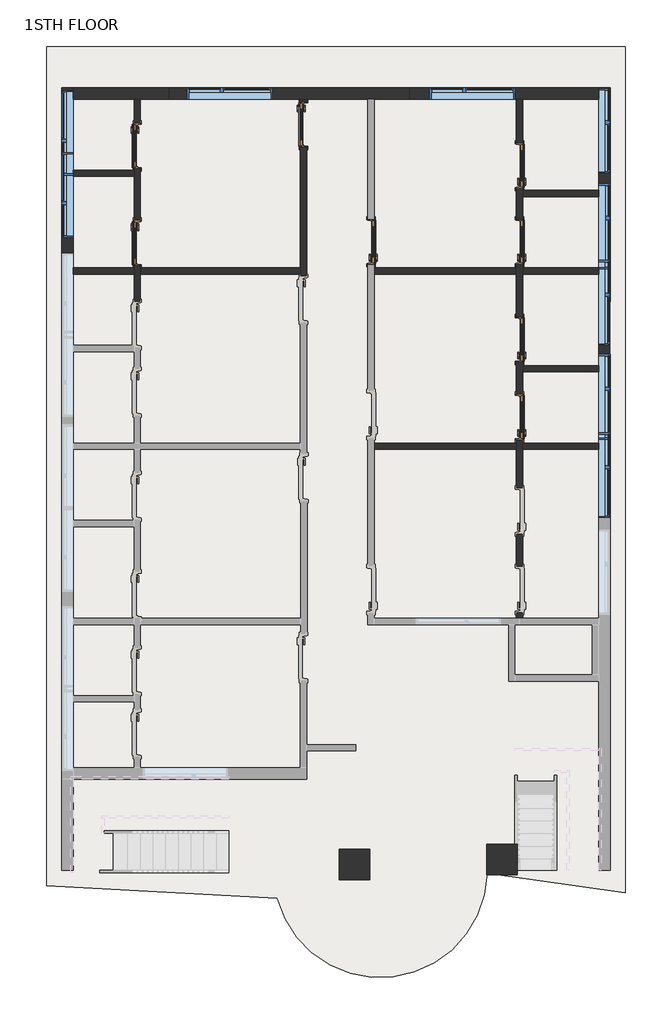
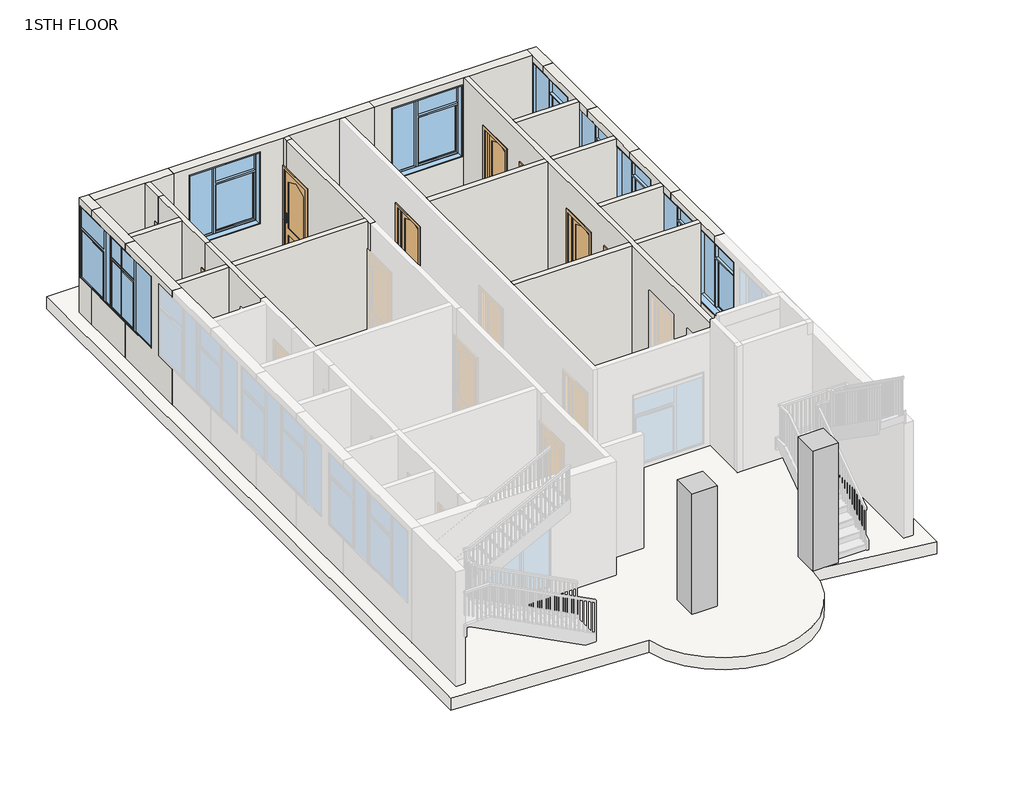
# One storey, part 2 of 4: 26 walls, 9 windows, 8 doors, 2 columns, 1 slab.
"""IFC4 building model written with IfcOpenShell, lengths in millimetres."""

from ifc_helpers import new_model, si_unit, point, frame, frame_2d, origin, place, context, project, spatial, polyline, circle_curve, trimmed, segment, composite_curve, outline, extrude, faceted_brep, transform, mapped, element, save
from components import column_8afb6978, door_346b4a94, m_window_casement_double_sidelight_1702_x_1829mm_c8b42c7f

model = new_model("IFC4")

# Units and contexts
model_context = context("Model", 3, world=origin())
ifc_project = project(units=[si_unit("LENGTHUNIT", "METRE", prefix="MILLI")], contexts=[model_context])

# Site, building, storey
site = spatial("IfcSite", under=ifc_project)
building = spatial("IfcBuilding", under=site)
storey = spatial("IfcBuildingStorey", under=building, Name="1STH FLOOR", Elevation=3200.4)

# Columns
placement = place(None, origin())
element("IfcColumn", 1, ObjectType="Rectangular Column : 24\" x 24\"", at=placement, inside=storey, context=model_context, shape_type="SweptSolid", body=[
    extrude(outline(polyline([(2657.4891134, -7132.8082131), (2657.4891134, -7742.4082131), (2047.8891134, -7742.4082131), (2047.8891134, -7132.8082131), (2657.4891134, -7132.8082131)])), frame((0.0, 0.0, 3200.4), z_axis=(0.0, 0.0, 1.0), x_axis=(1.0, 0.0, 0.0)), (0.0, 0.0, 1.0), 3048.0),
])
column_shape = column_8afb6978(model_context)
element("IfcColumn", 2, ObjectType="Rectangular Column : 24\" x 24\"", at=placement, inside=storey, context=model_context, shape_type="MappedRepresentation", body=[
    mapped(column_shape, transform((-606.4108866, -7539.2082131, 0.0), x_axis=(1.0, 0.0, 0.0), y_axis=(0.0, 1.0, 0.0), z_axis=(0.0, 0.0, 1.0))),
])

# Doors
door_shape = door_346b4a94(model_context)
element("IfcDoor", 3, ObjectType="2'10\"X7'", at=placement, inside=storey, context=model_context, shape_type="MappedRepresentation", body=[
    mapped(door_shape, transform((2698.7641134, 6449.4399728, 3200.4), x_axis=(0.0, -1.0, 0.0), y_axis=(1.0, 0.0, 0.0), z_axis=(0.0, 0.0, 1.0))),
])
element("IfcDoor", 4, ObjectType="2'10\"X7'", at=placement, inside=storey, context=model_context, shape_type="MappedRepresentation", body=[
    mapped(door_shape, transform((2698.7641134, 4925.4399728, 3200.4), x_axis=(0.0, -1.0, 0.0), y_axis=(1.0, 0.0, 0.0), z_axis=(0.0, 0.0, 1.0))),
])
element("IfcDoor", 5, ObjectType="2'10\"X7'", at=placement, inside=storey, context=model_context, shape_type="MappedRepresentation", body=[
    mapped(door_shape, transform((2698.7641134, 2969.6399728, 3200.4), x_axis=(0.0, -1.0, 0.0), y_axis=(1.0, 0.0, 0.0), z_axis=(0.0, 0.0, 1.0))),
])
element("IfcDoor", 6, ObjectType="2'10\"X7'", at=placement, inside=storey, context=model_context, shape_type="MappedRepresentation", body=[
    mapped(door_shape, transform((2698.7641134, 1420.2399728, 3200.4), x_axis=(0.0, -1.0, 0.0), y_axis=(1.0, 0.0, 0.0), z_axis=(0.0, 0.0, 1.0))),
])
element("IfcDoor", 7, ObjectType="2'10\"X7'", at=placement, inside=storey, context=model_context, shape_type="MappedRepresentation", body=[
    mapped(door_shape, transform((-273.0358866, 4925.4399728, 3200.4), x_axis=(0.0, -1.0, 0.0), y_axis=(1.0, 0.0, 0.0), z_axis=(0.0, 0.0, 1.0))),
])
element("IfcDoor", 8, ObjectType="2'10\"X7'", at=placement, inside=storey, context=model_context, shape_type="MappedRepresentation", body=[
    mapped(door_shape, transform((-4952.9858866, 4900.320652, 3200.4), x_axis=(0.0, 1.0, 0.0), y_axis=(-1.0, 0.0, 0.0), z_axis=(0.0, 0.0, 1.0))),
])
element("IfcDoor", 9, ObjectType="2'10\"X7'", at=placement, inside=storey, context=model_context, shape_type="MappedRepresentation", body=[
    mapped(door_shape, transform((-4952.9858866, 6843.9929737, 3200.4), x_axis=(0.0, 1.0, 0.0), y_axis=(-1.0, 0.0, 0.0), z_axis=(0.0, 0.0, 1.0))),
])
element("IfcDoor", 10, ObjectType="2'10\"X7'", at=placement, inside=storey, context=model_context, shape_type="MappedRepresentation", body=[
    mapped(door_shape, transform((-1625.5858866, 7274.3310623, 3200.4), x_axis=(0.0, 1.0, 0.0), y_axis=(-1.0, 0.0, 0.0), z_axis=(0.0, 0.0, 1.0))),
])

# Slab
element("IfcSlab", 11, ObjectType="Generic - 12\"", at=placement, inside=storey, context=model_context, shape_type="SweptSolid", body=[
    extrude(outline(composite_curve([segment(polyline([(4815.1311655, 8833.6177996), (4815.1311655, -8095.4822004), (2048.5236178, -7706.6608663)]), True, "CONTINUOUS"), segment(trimmed(circle_curve(frame_2d((-85.9459984, -7660.7851902)), 2134.962557), [point((2048.5236178, -7706.6608663))], [point((-2148.0488767, -8213.7741944))], False, "CARTESIAN"), True, "CONTINUOUS"), segment(polyline([(-2148.0488767, -8213.7741944), (-6765.9108866, -7964.6582131), (-6765.9108866, 8833.6177996), (4815.1311655, 8833.6177996)]), True, "CONTINUOUS")], self_intersect=False)), frame((0.0, 0.0, 2895.6), z_axis=(0.0, 0.0, 1.0), x_axis=(1.0, 0.0, 0.0)), (0.0, 0.0, 1.0), 304.8),
])

# Walls
element("IfcWall", 12, ObjectType="Generic - 4.5\"", at=placement, inside=storey, context=model_context, shape_type="SweptSolid", body=[
    extrude(outline(polyline([(7782.9399728, 6096.0), (7782.9399728, 3200.4), (7300.7929737, 3200.4), (7300.7929737, 5359.0), (7224.9929737, 5359.0), (7224.9929737, 6096.0), (7782.9399728, 6096.0)])), frame((-5013.3108866, 0.0, 0.0), z_axis=(1.0, 0.0, 0.0), x_axis=(0.0, 1.0, 0.0)), (0.0, 0.0, 1.0), 127.0),
])
element("IfcWall", 13, ObjectType="Generic - 4.5\"", at=placement, inside=storey, context=model_context, shape_type="Brep", body=[
    faceted_brep([(-5013.3108866, 5281.320652, 5359.0), (-5013.3108866, 5281.320652, 6096.0), (-5013.3108866, 6233.5399728, 6096.0), (-5013.3108866, 6360.5399728, 6096.0), (-5013.3108866, 7224.9929737, 6096.0), (-5013.3108866, 7224.9929737, 5359.0), (-5013.3108866, 6387.1929737, 5359.0), (-5013.3108866, 6387.1929737, 3200.4), (-5013.3108866, 6360.5399728, 3200.4), (-5013.3108866, 6233.5399728, 3200.4), (-5013.3108866, 5357.120652, 3200.4), (-5013.3108866, 5357.120652, 5359.0), (-4886.3108866, 5281.320652, 6096.0), (-4886.3108866, 5281.320652, 5359.0), (-4886.3108866, 5357.120652, 5359.0), (-4886.3108866, 5357.120652, 3200.4), (-4886.3108866, 6387.1929737, 3200.4), (-4886.3108866, 6387.1929737, 5359.0), (-4886.3108866, 7224.9929737, 5359.0), (-4886.3108866, 7224.9929737, 6096.0)], [[[0, 1, 2, 3, 4, 5, 6, 7, 8, 9, 10, 11]], [[12, 13, 14, 15, 16, 17, 18, 19]], [[15, 10, 9, 8, 7, 16]], [[1, 0, 13, 12]], [[4, 19, 18, 5]], [[14, 11, 10, 15]], [[11, 14, 13, 0]], [[17, 6, 5, 18]], [[6, 17, 16, 7]], [[4, 3, 2, 1, 12, 19]]]),
])
element("IfcWall", 14, ObjectType="Generic - 4.5\"", at=placement, inside=storey, context=model_context, shape_type="SweptSolid", body=[
    extrude(outline(polyline([(-5013.3108866, 6233.5399728), (-6232.5508078, 6233.5399728), (-6232.5508078, 6360.5399728), (-5013.3108866, 6360.5399728), (-5013.3108866, 6233.5399728)])), frame((0.0, 0.0, 3200.4), z_axis=(0.0, 0.0, 1.0), x_axis=(1.0, 0.0, 0.0)), (0.0, 0.0, 1.0), 2895.6),
])
element("IfcWall", 15, ObjectType="Generic - 4.5\"", at=placement, inside=storey, context=model_context, shape_type="SweptSolid", body=[
    extrude(outline(polyline([(-5013.3108866, 4277.7399728), (-6232.5508078, 4277.7399728), (-6232.5508078, 4404.7399728), (-5013.3108866, 4404.7399728), (-5013.3108866, 4277.7399728)])), frame((0.0, 0.0, 3200.4), z_axis=(0.0, 0.0, 1.0), x_axis=(1.0, 0.0, 0.0)), (0.0, 0.0, 1.0), 2895.6),
])
element("IfcWall", 16, ObjectType="Generic - 4.5\"", at=placement, inside=storey, context=model_context, shape_type="Brep", body=[
    faceted_brep([(-5013.3108866, 2968.8174518, 5359.0), (-5013.3108866, 2968.8174518, 6096.0), (-5013.3108866, 4277.7399728, 6096.0), (-5013.3108866, 4404.7399728, 6096.0), (-5013.3108866, 5281.320652, 6096.0), (-5013.3108866, 5281.320652, 5359.0), (-5013.3108866, 4443.520652, 5359.0), (-5013.3108866, 4443.520652, 3200.4), (-5013.3108866, 4404.7399728, 3200.4), (-5013.3108866, 4277.7399728, 3200.4), (-5013.3108866, 3730.4174518, 3200.4), (-5013.3108866, 3730.4174518, 5359.0), (-4886.3108866, 2968.8174518, 6096.0), (-4886.3108866, 2968.8174518, 5359.0), (-4886.3108866, 3730.4174518, 5359.0), (-4886.3108866, 3730.4174518, 3200.4), (-4886.3108866, 4277.7399728, 3200.4), (-4886.3108866, 4404.7399728, 3200.4), (-4886.3108866, 4443.520652, 3200.4), (-4886.3108866, 4443.520652, 5359.0), (-4886.3108866, 5281.320652, 5359.0), (-4886.3108866, 5281.320652, 6096.0), (-4886.3108866, 4404.7399728, 6096.0), (-4886.3108866, 4277.7399728, 6096.0)], [[[0, 1, 2, 3, 4, 5, 6, 7, 8, 9, 10, 11]], [[12, 13, 14, 15, 16, 17, 18, 19, 20, 21, 22, 23]], [[15, 10, 9, 8, 7, 18, 17, 16]], [[1, 0, 13, 12]], [[4, 21, 20, 5]], [[14, 11, 10, 15]], [[11, 14, 13, 0]], [[19, 6, 5, 20]], [[6, 19, 18, 7]], [[4, 3, 2, 1, 12, 23, 22, 21]]]),
])
element("IfcWall", 17, ObjectType="Generic - 4.5\"", at=placement, inside=storey, context=model_context, shape_type="SweptSolid", body=[
    extrude(outline(polyline([(-1685.9108866, 4277.7399728), (-4886.3108866, 4277.7399728), (-4886.3108866, 4404.7399728), (-1685.9108866, 4404.7399728), (-1685.9108866, 4277.7399728)])), frame((0.0, 0.0, 3200.4), z_axis=(0.0, 0.0, 1.0), x_axis=(1.0, 0.0, 0.0)), (0.0, 0.0, 1.0), 2895.6),
])
element("IfcWall", 18, ObjectType="Generic - 4.5\"", at=placement, inside=storey, context=model_context, shape_type="SweptSolid", body=[
    extrude(outline(polyline([(7782.9399728, 6096.0), (7782.9399728, 3200.4), (7731.1310623, 3200.4), (7731.1310623, 5359.0), (7655.3310623, 5359.0), (7655.3310623, 6096.0), (7782.9399728, 6096.0)])), frame((-1685.9108866, 0.0, 0.0), z_axis=(1.0, 0.0, 0.0), x_axis=(0.0, 1.0, 0.0)), (0.0, 0.0, 1.0), 127.0),
])
element("IfcWall", 19, ObjectType="Generic - 4.5\"", at=placement, inside=storey, context=model_context, shape_type="Brep", body=[
    faceted_brep([(-1685.9108866, 4182.2008884, 5359.0), (-1685.9108866, 4182.2008884, 6096.0), (-1685.9108866, 4277.7399728, 6096.0), (-1685.9108866, 4404.7399728, 6096.0), (-1685.9108866, 7655.3310623, 6096.0), (-1685.9108866, 7655.3310623, 5359.0), (-1685.9108866, 6817.5310623, 5359.0), (-1685.9108866, 6817.5310623, 3200.4), (-1685.9108866, 4404.7399728, 3200.4), (-1685.9108866, 4277.7399728, 3200.4), (-1685.9108866, 4232.6008884, 3200.4), (-1685.9108866, 4232.6008884, 5359.0), (-1558.9108866, 4182.2008884, 6096.0), (-1558.9108866, 4182.2008884, 5359.0), (-1558.9108866, 4232.6008884, 5359.0), (-1558.9108866, 4232.6008884, 3200.4), (-1558.9108866, 6817.5310623, 3200.4), (-1558.9108866, 6817.5310623, 5359.0), (-1558.9108866, 7655.3310623, 5359.0), (-1558.9108866, 7655.3310623, 6096.0), (-1685.4871817, 4182.2008884, 5359.0), (-1685.4871817, 4182.2008884, 6096.0)], [[[0, 1, 2, 3, 4, 5, 6, 7, 8, 9, 10, 11]], [[12, 13, 14, 15, 16, 17, 18, 19]], [[15, 10, 9, 8, 7, 16]], [[1, 0, 20, 13, 12, 21]], [[4, 19, 18, 5]], [[14, 11, 10, 15]], [[11, 14, 13, 20, 0]], [[17, 6, 5, 18]], [[6, 17, 16, 7]], [[4, 3, 2, 1, 21, 12, 19]]]),
])
element("IfcWall", 20, ObjectType="Generic - 4.5\"", at=placement, inside=storey, context=model_context, shape_type="Brep", body=[
    faceted_brep([(2632.0891134, 7782.9399728, 6096.0), (2632.0891134, 7782.9399728, 3200.4), (2632.0891134, 6906.2399728, 3200.4), (2632.0891134, 6906.2399728, 5359.0), (2632.0891134, 5992.6399728, 5359.0), (2632.0891134, 5992.6399728, 3200.4), (2632.0891134, 5382.2399728, 3200.4), (2632.0891134, 5382.2399728, 5359.0), (2632.0891134, 4468.6399728, 5359.0), (2632.0891134, 4468.6399728, 3200.4), (2632.0891134, 4404.7399728, 3200.4), (2632.0891134, 4277.7399728, 3200.4), (2632.0891134, 3426.4399728, 3200.4), (2632.0891134, 3426.4399728, 5359.0), (2632.0891134, 2512.8399728, 5359.0), (2632.0891134, 2512.8399728, 3200.4), (2632.0891134, 1877.0399728, 3200.4), (2632.0891134, 1877.0399728, 5359.0), (2632.0891134, 963.4399728, 5359.0), (2632.0891134, 963.4399728, 3200.4), (2632.0891134, 899.5399728, 3200.4), (2632.0891134, 772.5399728, 3200.4), (2632.0891134, -2.5600272, 3200.4), (2632.0891134, -2.5600272, 5359.0), (2632.0891134, -916.1600272, 5359.0), (2632.0891134, -916.1600272, 3200.4), (2632.0891134, -1577.3600272, 3200.4), (2632.0891134, -1577.3600272, 5359.0), (2632.0891134, -2490.9600272, 5359.0), (2632.0891134, -2490.9600272, 3200.4), (2632.0891134, -2605.6600272, 3200.4), (2632.0891134, -2605.6600272, 6096.0), (2632.0891134, 772.5399728, 6096.0), (2632.0891134, 899.5399728, 6096.0), (2632.0891134, 4277.7399728, 6096.0), (2632.0891134, 4404.7399728, 6096.0), (2759.0891134, 7782.9399728, 3200.4), (2759.0891134, 7782.9399728, 6096.0), (2759.0891134, 5954.1399728, 6096.0), (2759.0891134, 5827.1399728, 6096.0), (2759.0891134, 4404.7399728, 6096.0), (2759.0891134, 4277.7399728, 6096.0), (2759.0891134, 2448.9399728, 6096.0), (2759.0891134, 2321.9399728, 6096.0), (2759.0891134, 899.5399728, 6096.0), (2759.0891134, 772.5399728, 6096.0), (2759.0891134, -2605.6600272, 6096.0), (2759.0891134, -2605.6600272, 3200.4), (2759.0891134, -2490.9600272, 3200.4), (2759.0891134, -2490.9600272, 5359.0), (2759.0891134, -1577.3600272, 5359.0), (2759.0891134, -1577.3600272, 3200.4), (2759.0891134, -916.1600272, 3200.4), (2759.0891134, -916.1600272, 5359.0), (2759.0891134, -2.5600272, 5359.0), (2759.0891134, -2.5600272, 3200.4), (2759.0891134, 772.5399728, 3200.4), (2759.0891134, 899.5399728, 3200.4), (2759.0891134, 963.4399728, 3200.4), (2759.0891134, 963.4399728, 5359.0), (2759.0891134, 1877.0399728, 5359.0), (2759.0891134, 1877.0399728, 3200.4), (2759.0891134, 2321.9399728, 3200.4), (2759.0891134, 2448.9399728, 3200.4), (2759.0891134, 2512.8399728, 3200.4), (2759.0891134, 2512.8399728, 5359.0), (2759.0891134, 3426.4399728, 5359.0), (2759.0891134, 3426.4399728, 3200.4), (2759.0891134, 4277.7399728, 3200.4), (2759.0891134, 4404.7399728, 3200.4), (2759.0891134, 4468.6399728, 3200.4), (2759.0891134, 4468.6399728, 5359.0), (2759.0891134, 5382.2399728, 5359.0), (2759.0891134, 5382.2399728, 3200.4), (2759.0891134, 5827.1399728, 3200.4), (2759.0891134, 5954.1399728, 3200.4), (2759.0891134, 5992.6399728, 3200.4), (2759.0891134, 5992.6399728, 5359.0), (2759.0891134, 6906.2399728, 5359.0), (2759.0891134, 6906.2399728, 3200.4), (2695.5891134, -2605.6600272, 3200.4), (2695.5891134, -2605.6600272, 6096.0)], [[[0, 1, 2, 3, 4, 5, 6, 7, 8, 9, 10, 11, 12, 13, 14, 15, 16, 17, 18, 19, 20, 21, 22, 23, 24, 25, 26, 27, 28, 29, 30, 31, 32, 33, 34, 35]], [[36, 37, 38, 39, 40, 41, 42, 43, 44, 45, 46, 47, 48, 49, 50, 51, 52, 53, 54, 55, 56, 57, 58, 59, 60, 61, 62, 63, 64, 65, 66, 67, 68, 69, 70, 71, 72, 73, 74, 75, 76, 77, 78, 79]], [[1, 36, 79, 2]], [[5, 76, 75, 74, 73, 6]], [[9, 70, 69, 68, 67, 12, 11, 10]], [[15, 64, 63, 62, 61, 16]], [[19, 58, 57, 56, 55, 22, 21, 20]], [[25, 52, 51, 26]], [[47, 80, 30, 29, 48]], [[1, 0, 37, 36]], [[31, 30, 80, 47, 46, 81]], [[4, 77, 76, 5]], [[77, 4, 3, 78]], [[78, 3, 2, 79]], [[9, 8, 71, 70]], [[8, 7, 72, 71]], [[7, 6, 73, 72]], [[14, 65, 64, 15]], [[65, 14, 13, 66]], [[66, 13, 12, 67]], [[18, 59, 58, 19]], [[59, 18, 17, 60]], [[60, 17, 16, 61]], [[24, 53, 52, 25]], [[53, 24, 23, 54]], [[54, 23, 22, 55]], [[28, 49, 48, 29]], [[49, 28, 27, 50]], [[50, 27, 26, 51]], [[0, 35, 34, 33, 32, 31, 81, 46, 45, 44, 43, 42, 41, 40, 39, 38, 37]]]),
])
element("IfcWall", 21, ObjectType="Generic - 4.5\"", at=placement, inside=storey, context=model_context, shape_type="SweptSolid", body=[
    extrude(outline(polyline([(2632.0891134, 4277.7399728), (-212.7108866, 4277.7399728), (-212.7108866, 4404.7399728), (2632.0891134, 4404.7399728), (2632.0891134, 4277.7399728)])), frame((0.0, 0.0, 3200.4), z_axis=(0.0, 0.0, 1.0), x_axis=(1.0, 0.0, 0.0)), (0.0, 0.0, 1.0), 2895.6),
])
element("IfcWall", 22, ObjectType="Generic - 4.5\"", at=placement, inside=storey, context=model_context, shape_type="SweptSolid", body=[
    extrude(outline(polyline([(2632.0891134, 772.5399728), (-212.7108866, 772.5399728), (-212.7108866, 899.5399728), (2632.0891134, 899.5399728), (2632.0891134, 772.5399728)])), frame((0.0, 0.0, 3200.4), z_axis=(0.0, 0.0, 1.0), x_axis=(1.0, 0.0, 0.0)), (0.0, 0.0, 1.0), 2895.6),
])
element("IfcWall", 23, ObjectType="Generic - 4.5\"", at=placement, inside=storey, context=model_context, shape_type="SweptSolid", body=[
    extrude(outline(polyline([(4281.587404, 5827.1399728), (2759.0891134, 5827.1399728), (2759.0891134, 5954.1399728), (4281.587404, 5954.1399728), (4281.587404, 5827.1399728)])), frame((0.0, 0.0, 3200.4), z_axis=(0.0, 0.0, 1.0), x_axis=(1.0, 0.0, 0.0)), (0.0, 0.0, 1.0), 2895.6),
])
element("IfcWall", 24, ObjectType="Generic - 4.5\"", at=placement, inside=storey, context=model_context, shape_type="SweptSolid", body=[
    extrude(outline(polyline([(4283.9989713, 4277.7399728), (2759.0891134, 4277.7399728), (2759.0891134, 4404.7399728), (4283.9989713, 4404.7399728), (4283.9989713, 4277.7399728)])), frame((0.0, 0.0, 3200.4), z_axis=(0.0, 0.0, 1.0), x_axis=(1.0, 0.0, 0.0)), (0.0, 0.0, 1.0), 2895.6),
])
element("IfcWall", 25, ObjectType="Generic - 4.5\"", at=placement, inside=storey, context=model_context, shape_type="SweptSolid", body=[
    extrude(outline(polyline([(4281.0767915, 2321.9399728), (2759.0891134, 2321.9399728), (2759.0891134, 2448.9399728), (4281.0767915, 2448.9399728), (4281.0767915, 2321.9399728)])), frame((0.0, 0.0, 3200.4), z_axis=(0.0, 0.0, 1.0), x_axis=(1.0, 0.0, 0.0)), (0.0, 0.0, 1.0), 2895.6),
])
element("IfcWall", 26, ObjectType="Generic - 4.5\"", at=placement, inside=storey, context=model_context, shape_type="SweptSolid", body=[
    extrude(outline(polyline([(4283.0918814, 772.5399728), (2759.0891134, 772.5399728), (2759.0891134, 899.5399728), (4283.0918814, 899.5399728), (4283.0918814, 772.5399728)])), frame((0.0, 0.0, 3200.4), z_axis=(0.0, 0.0, 1.0), x_axis=(1.0, 0.0, 0.0)), (0.0, 0.0, 1.0), 2895.6),
])
element("IfcWall", 27, ObjectType="Generic - 9\"", at=placement, inside=storey, context=model_context, shape_type="Brep", body=[
    faceted_brep([(-6232.5108866, 7782.9399728, 3200.4), (-5013.3108866, 7782.9399728, 3200.4), (-4886.3108866, 7782.9399728, 3200.4), (-4318.2603585, 7782.9399728, 3200.4), (-4318.2603585, 7782.9399728, 6096.0), (-4886.3108866, 7782.9399728, 6096.0), (-5013.3108866, 7782.9399728, 6096.0), (-6232.5108866, 7782.9399728, 6096.0), (-6232.5108866, 8011.5399728, 3200.4), (-6232.5108866, 8011.5399728, 6096.0), (-4318.2603585, 8011.5399728, 6096.0), (-4318.2603585, 8011.5399728, 3200.4)], [[[0, 1, 2, 3, 4, 5, 6, 7]], [[8, 9, 10, 11]], [[3, 2, 1, 0, 8, 11]], [[4, 3, 11, 10]], [[0, 7, 9, 8]], [[7, 6, 5, 4, 10, 9]]]),
])
element("IfcWall", 28, ObjectType="Generic - 9\"", at=placement, inside=storey, context=model_context, shape_type="Brep", body=[
    faceted_brep([(-4318.2603585, 7782.9399728, 3200.4), (-1685.9108866, 7782.9399728, 3200.4), (-1558.9108866, 7782.9399728, 3200.4), (-339.7108866, 7782.9399728, 3200.4), (-212.7108866, 7782.9399728, 3200.4), (496.3553976, 7782.9399728, 3200.4), (496.3553976, 7782.9399728, 6096.0), (-212.7108866, 7782.9399728, 6096.0), (-339.7108866, 7782.9399728, 6096.0), (-1558.9108866, 7782.9399728, 6096.0), (-1685.9108866, 7782.9399728, 6096.0), (-4318.2603585, 7782.9399728, 6096.0), (-2248.1603585, 7782.9399728, 5929.2), (-2248.1603585, 7782.9399728, 4100.4), (-3949.9603585, 7782.9399728, 4100.4), (-3949.9603585, 7782.9399728, 5929.2), (-4318.2603585, 8011.5399728, 3200.4), (-4318.2603585, 8011.5399728, 6096.0), (496.3553976, 8011.5399728, 6096.0), (496.3553976, 8011.5399728, 3200.4), (-2248.1603585, 8011.5399728, 5929.2), (-3949.9603585, 8011.5399728, 5929.2), (-3949.9603585, 8011.5399728, 4100.4), (-2248.1603585, 8011.5399728, 4100.4)], [[[0, 1, 2, 3, 4, 5, 6, 7, 8, 9, 10, 11], [12, 13, 14, 15]], [[16, 17, 18, 19], [20, 21, 22, 23]], [[5, 4, 3, 2, 1, 0, 16, 19]], [[6, 5, 19, 18]], [[0, 11, 17, 16]], [[13, 12, 20, 23]], [[14, 13, 23, 22]], [[15, 14, 22, 21]], [[12, 15, 21, 20]], [[11, 10, 9, 8, 7, 6, 18, 17]]]),
])
element("IfcWall", 29, ObjectType="Generic - 9\"", at=placement, inside=storey, context=model_context, shape_type="Brep", body=[
    faceted_brep([(496.3553976, 7782.9399728, 3200.4), (2632.0891134, 7782.9399728, 3200.4), (2759.0891134, 7782.9399728, 3200.4), (4283.0891134, 7782.9399728, 3200.4), (4283.0891134, 7782.9399728, 6096.0), (2759.0891134, 7782.9399728, 6096.0), (2632.0891134, 7782.9399728, 6096.0), (496.3553976, 7782.9399728, 6096.0), (2606.6891134, 7782.9399728, 5929.2), (2606.6891134, 7782.9399728, 4100.4), (904.8891134, 7782.9399728, 4100.4), (904.8891134, 7782.9399728, 5929.2), (496.3553976, 8011.5399728, 3200.4), (496.3553976, 8011.5399728, 6096.0), (4283.0891134, 8011.5399728, 6096.0), (4283.0891134, 8011.5399728, 3200.4), (2606.6891134, 8011.5399728, 5929.2), (904.8891134, 8011.5399728, 5929.2), (904.8891134, 8011.5399728, 4100.4), (2606.6891134, 8011.5399728, 4100.4)], [[[0, 1, 2, 3, 4, 5, 6, 7], [8, 9, 10, 11]], [[12, 13, 14, 15], [16, 17, 18, 19]], [[3, 2, 1, 0, 12, 15]], [[0, 7, 13, 12]], [[9, 8, 16, 19]], [[10, 9, 19, 18]], [[11, 10, 18, 17]], [[8, 11, 17, 16]], [[4, 3, 15, 14]], [[7, 6, 5, 4, 14, 13]]]),
])
element("IfcWall", 30, ObjectType="Generic - 9\"", at=placement, inside=storey, context=model_context, shape_type="Brep", body=[
    faceted_brep([(4283.0891134, 8011.5399728, 3200.4), (4283.0891134, 7782.9399728, 3200.4), (4283.0891134, 7325.7399728, 3200.4), (4283.0891134, 7325.7399728, 4100.4), (4283.0891134, 7998.8399728, 4100.4), (4283.0891134, 7998.8399728, 5929.2), (4283.0891134, 7325.7399728, 5929.2), (4283.0891134, 7325.7399728, 6096.0), (4283.0891134, 7782.9399728, 6096.0), (4283.0891134, 8011.5399728, 6096.0), (4511.6891134, 7325.7399728, 3200.4), (4511.6891134, 8011.5399728, 3200.4), (4511.6891134, 8011.5399728, 6096.0), (4511.6891134, 7325.7399728, 6096.0), (4511.6891134, 7325.7399728, 5929.2), (4511.6891134, 7998.8399728, 5929.2), (4511.6891134, 7998.8399728, 4100.4), (4511.6891134, 7325.7399728, 4100.4), (4510.187404, 7325.7399728, 3200.4), (4510.187404, 7325.7399728, 4100.4), (4510.187404, 7325.7399728, 6096.0), (4510.187404, 7325.7399728, 5929.2)], [[[0, 1, 2, 3, 4, 5, 6, 7, 8, 9]], [[10, 11, 12, 13, 14, 15, 16, 17]], [[2, 1, 0, 11, 10, 18]], [[2, 18, 10, 17, 19, 3]], [[13, 20, 7, 6, 21, 14]], [[16, 4, 3, 19, 17]], [[4, 16, 15, 5]], [[5, 15, 14, 21, 6]], [[0, 9, 12, 11]], [[9, 8, 7, 20, 13, 12]]]),
])
element("IfcWall", 31, ObjectType="Generic - 9\"", at=placement, inside=storey, context=model_context, shape_type="Brep", body=[
    faceted_brep([(4281.587404, 7325.7399728, 3200.4), (4281.587404, 5954.1399728, 3200.4), (4281.587404, 5827.1399728, 3200.4), (4281.587404, 5490.9915892, 3200.4), (4281.587404, 5490.9915892, 4100.4), (4281.587404, 6087.8915892, 4100.4), (4281.587404, 6087.8915892, 5929.2), (4281.587404, 5490.9915892, 5929.2), (4281.587404, 5490.9915892, 6096.0), (4281.587404, 5827.1399728, 6096.0), (4281.587404, 5954.1399728, 6096.0), (4281.587404, 7325.7399728, 6096.0), (4281.587404, 7325.7399728, 5929.2), (4281.587404, 6297.0399728, 5929.2), (4281.587404, 6297.0399728, 4100.4), (4281.587404, 7325.7399728, 4100.4), (4510.187404, 5490.9915892, 3200.4), (4510.187404, 7325.7399728, 3200.4), (4510.187404, 7325.7399728, 4100.4), (4510.187404, 6297.0399728, 4100.4), (4510.187404, 6297.0399728, 5929.2), (4510.187404, 7325.7399728, 5929.2), (4510.187404, 7325.7399728, 6096.0), (4510.187404, 5490.9915892, 6096.0), (4510.187404, 5490.9915892, 5929.2), (4510.187404, 6087.8915892, 5929.2), (4510.187404, 6087.8915892, 4100.4), (4510.187404, 5490.9915892, 4100.4), (4283.0891134, 7325.7399728, 3200.4), (4283.9989713, 5490.9915892, 3200.4), (4283.9989713, 5490.9915892, 4100.4), (4283.9989713, 5490.9915892, 6096.0), (4283.9989713, 5490.9915892, 5929.2), (4283.0891134, 7325.7399728, 4100.4), (4283.0891134, 7325.7399728, 6096.0), (4283.0891134, 7325.7399728, 5929.2)], [[[0, 1, 2, 3, 4, 5, 6, 7, 8, 9, 10, 11, 12, 13, 14, 15]], [[16, 17, 18, 19, 20, 21, 22, 23, 24, 25, 26, 27]], [[3, 2, 1, 0, 28, 17, 16, 29]], [[3, 29, 16, 27, 30, 4]], [[23, 31, 8, 7, 32, 24]], [[17, 28, 0, 15, 33, 18]], [[12, 11, 34, 22, 21, 35]], [[13, 20, 19, 14]], [[14, 19, 18, 33, 15]], [[20, 13, 12, 35, 21]], [[26, 5, 4, 30, 27]], [[5, 26, 25, 6]], [[6, 25, 24, 32, 7]], [[11, 10, 9, 8, 31, 23, 22, 34]]]),
])
element("IfcWall", 32, ObjectType="Generic - 9\"", at=placement, inside=storey, context=model_context, shape_type="Brep", body=[
    faceted_brep([(4283.9989713, 5490.9915892, 3200.4), (4283.9989713, 4404.7399728, 3200.4), (4283.9989713, 4277.7399728, 3200.4), (4283.9989713, 3730.8359967, 3200.4), (4283.9989713, 3730.8359967, 4100.4), (4283.9989713, 5490.9915892, 4100.4), (4512.5989713, 3730.8359967, 3200.4), (4512.5989713, 5490.9915892, 3200.4), (4512.5989713, 5490.9915892, 4100.4), (4512.5989713, 3730.8359967, 4100.4), (4510.187404, 5490.9915892, 3200.4), (4509.6767915, 3730.8359967, 3200.4), (4509.6767915, 3730.8359967, 4100.4), (4510.187404, 5490.9915892, 4100.4)], [[[0, 1, 2, 3, 4, 5]], [[6, 7, 8, 9]], [[3, 2, 1, 0, 10, 7, 6, 11]], [[3, 11, 6, 9, 12, 4]], [[7, 10, 0, 5, 13, 8]], [[8, 13, 5, 4, 12, 9]]]),
    faceted_brep([(4283.9989713, 5490.9915892, 6096.0), (4283.9989713, 5490.9915892, 5929.2), (4283.9989713, 3730.8359967, 5929.2), (4283.9989713, 3730.8359967, 6096.0), (4283.9989713, 4277.7399728, 6096.0), (4283.9989713, 4404.7399728, 6096.0), (4512.5989713, 3730.8359967, 5929.2), (4512.5989713, 5490.9915892, 5929.2), (4512.5989713, 5490.9915892, 6096.0), (4512.5989713, 3730.8359967, 6096.0), (4509.6767915, 3730.8359967, 6096.0), (4509.6767915, 3730.8359967, 5929.2), (4510.187404, 5490.9915892, 6096.0), (4510.187404, 5490.9915892, 5929.2)], [[[0, 1, 2, 3, 4, 5]], [[6, 7, 8, 9]], [[9, 10, 3, 2, 11, 6]], [[1, 0, 12, 8, 7, 13]], [[1, 13, 7, 6, 11, 2]], [[0, 5, 4, 3, 10, 9, 8, 12]]]),
])
element("IfcWall", 33, ObjectType="Generic - 9\"", at=placement, inside=storey, context=model_context, shape_type="Brep", body=[
    faceted_brep([(4281.0767915, 3730.8359967, 3200.4), (4281.0767915, 2448.9399728, 3200.4), (4281.0767915, 2321.9399728, 3200.4), (4281.0767915, 2023.9001312, 3200.4), (4281.0767915, 2023.9001312, 4100.4), (4281.0767915, 2671.6001312, 4100.4), (4281.0767915, 2671.6001312, 5929.2), (4281.0767915, 2023.9001312, 5929.2), (4281.0767915, 2023.9001312, 6096.0), (4281.0767915, 2321.9399728, 6096.0), (4281.0767915, 2448.9399728, 6096.0), (4281.0767915, 3730.8359967, 6096.0), (4281.0767915, 3730.8359967, 5929.2), (4281.0767915, 2854.5359967, 5929.2), (4281.0767915, 2854.5359967, 4100.4), (4281.0767915, 3730.8359967, 4100.4), (4509.6767915, 2023.9001312, 3200.4), (4509.6767915, 3730.8359967, 3200.4), (4509.6767915, 3730.8359967, 4100.4), (4509.6767915, 2854.5359967, 4100.4), (4509.6767915, 2854.5359967, 5929.2), (4509.6767915, 3730.8359967, 5929.2), (4509.6767915, 3730.8359967, 6096.0), (4509.6767915, 2023.9001312, 6096.0), (4509.6767915, 2023.9001312, 5929.2), (4509.6767915, 2671.6001312, 5929.2), (4509.6767915, 2671.6001312, 4100.4), (4509.6767915, 2023.9001312, 4100.4), (4283.9989713, 3730.8359967, 3200.4), (4283.0918814, 2023.9001312, 3200.4), (4283.0918814, 2023.9001312, 4100.4), (4283.0918814, 2023.9001312, 6096.0), (4283.0918814, 2023.9001312, 5929.2), (4283.9989713, 3730.8359967, 4100.4), (4283.9989713, 3730.8359967, 6096.0), (4283.9989713, 3730.8359967, 5929.2)], [[[0, 1, 2, 3, 4, 5, 6, 7, 8, 9, 10, 11, 12, 13, 14, 15]], [[16, 17, 18, 19, 20, 21, 22, 23, 24, 25, 26, 27]], [[3, 2, 1, 0, 28, 17, 16, 29]], [[3, 29, 16, 27, 30, 4]], [[23, 31, 8, 7, 32, 24]], [[17, 28, 0, 15, 33, 18]], [[12, 11, 34, 22, 21, 35]], [[13, 20, 19, 14]], [[14, 19, 18, 33, 15]], [[20, 13, 12, 35, 21]], [[26, 5, 4, 30, 27]], [[5, 26, 25, 6]], [[6, 25, 24, 32, 7]], [[11, 10, 9, 8, 31, 23, 22, 34]]]),
])
element("IfcWall", 34, ObjectType="Generic - 9\"", at=placement, inside=storey, context=model_context, shape_type="Brep", body=[
    faceted_brep([(4283.0918814, 2023.9001312, 3200.4), (4283.0918814, 899.5399728, 3200.4), (4283.0918814, 772.5399728, 3200.4), (4283.0918814, 200.5184135, 3200.4), (4283.0918814, 200.5184135, 4100.4), (4283.0918814, 2023.9001312, 4100.4), (4511.6918814, 200.5184135, 3200.4), (4511.6918814, 2023.9001312, 3200.4), (4511.6918814, 2023.9001312, 4100.4), (4511.6918814, 200.5184135, 4100.4), (4509.6767915, 2023.9001312, 3200.4), (4510.3311655, 200.5184135, 3200.4), (4510.3311655, 200.5184135, 4100.4), (4509.6767915, 2023.9001312, 4100.4)], [[[0, 1, 2, 3, 4, 5]], [[6, 7, 8, 9]], [[3, 2, 1, 0, 10, 7, 6, 11]], [[3, 11, 6, 9, 12, 4]], [[7, 10, 0, 5, 13, 8]], [[8, 13, 5, 4, 12, 9]]]),
    faceted_brep([(4283.0918814, 2023.9001312, 6096.0), (4283.0918814, 2023.9001312, 5929.2), (4283.0918814, 200.5184135, 5929.2), (4283.0918814, 200.5184135, 6096.0), (4283.0918814, 772.5399728, 6096.0), (4283.0918814, 899.5399728, 6096.0), (4511.6918814, 200.5184135, 5929.2), (4511.6918814, 2023.9001312, 5929.2), (4511.6918814, 2023.9001312, 6096.0), (4511.6918814, 200.5184135, 6096.0), (4510.3311655, 200.5184135, 6096.0), (4510.3311655, 200.5184135, 5929.2), (4509.6767915, 2023.9001312, 6096.0), (4509.6767915, 2023.9001312, 5929.2)], [[[0, 1, 2, 3, 4, 5]], [[6, 7, 8, 9]], [[9, 10, 3, 2, 11, 6]], [[1, 0, 12, 8, 7, 13]], [[1, 13, 7, 6, 11, 2]], [[0, 5, 4, 3, 10, 9, 8, 12]]]),
])
element("IfcWall", 35, ObjectType="Generic - 9\"", at=placement, inside=storey, context=model_context, shape_type="Brep", body=[
    faceted_brep([(-6232.5508078, 4130.2388609, 3200.4), (-6232.5508078, 4277.7399728, 3200.4), (-6232.5508078, 4404.7399728, 3200.4), (-6232.5508078, 6088.0863192, 3200.4), (-6232.5508078, 6088.0863192, 4100.4), (-6232.5508078, 5008.5863192, 4100.4), (-6232.5508078, 5008.5863192, 5929.2), (-6232.5508078, 6088.0863192, 5929.2), (-6232.5508078, 6088.0863192, 6096.0), (-6232.5508078, 4404.7399728, 6096.0), (-6232.5508078, 4277.7399728, 6096.0), (-6232.5508078, 4130.2388609, 6096.0), (-6232.5508078, 4130.2388609, 5929.2), (-6232.5508078, 4701.7388609, 5929.2), (-6232.5508078, 4701.7388609, 4100.4), (-6232.5508078, 4130.2388609, 4100.4), (-6461.1508078, 6088.0863192, 3200.4), (-6461.1508078, 4130.2388609, 3200.4), (-6461.1508078, 4130.2388609, 4100.4), (-6461.1508078, 4701.7388609, 4100.4), (-6461.1508078, 4701.7388609, 5929.2), (-6461.1508078, 4130.2388609, 5929.2), (-6461.1508078, 4130.2388609, 6096.0), (-6461.1508078, 6088.0863192, 6096.0), (-6461.1508078, 6088.0863192, 5929.2), (-6461.1508078, 5008.5863192, 5929.2), (-6461.1508078, 5008.5863192, 4100.4), (-6461.1508078, 6088.0863192, 4100.4)], [[[0, 1, 2, 3, 4, 5, 6, 7, 8, 9, 10, 11, 12, 13, 14, 15]], [[16, 17, 18, 19, 20, 21, 22, 23, 24, 25, 26, 27]], [[3, 2, 1, 0, 17, 16]], [[3, 16, 27, 4]], [[8, 7, 24, 23]], [[17, 0, 15, 18]], [[11, 22, 21, 12]], [[26, 5, 4, 27]], [[5, 26, 25, 6]], [[6, 25, 24, 7]], [[13, 20, 19, 14]], [[14, 19, 18, 15]], [[20, 13, 12, 21]], [[11, 10, 9, 8, 23, 22]]]),
])
element("IfcWall", 36, ObjectType="Generic - 9\"", at=placement, inside=storey, context=model_context, shape_type="Brep", body=[
    faceted_brep([(-6232.5508078, 6088.0863192, 3200.4), (-6232.5508078, 6233.5399728, 3200.4), (-6232.5508078, 6360.5399728, 3200.4), (-6232.5508078, 7490.3748838, 3200.4), (-6232.5508078, 7490.3748838, 4100.4), (-6232.5508078, 6088.0863192, 4100.4), (-6461.1508078, 7490.3748838, 3200.4), (-6461.1508078, 6088.0863192, 3200.4), (-6461.1508078, 6088.0863192, 4100.4), (-6461.1508078, 7490.3748838, 4100.4)], [[[0, 1, 2, 3, 4, 5]], [[6, 7, 8, 9]], [[3, 2, 1, 0, 7, 6]], [[3, 6, 9, 4]], [[7, 0, 5, 8]], [[4, 9, 8, 5]]]),
    faceted_brep([(-6232.5508078, 6088.0863192, 5929.2), (-6232.5508078, 7490.3748838, 5929.2), (-6232.5508078, 7490.3748838, 6096.0), (-6232.5508078, 6360.5399728, 6096.0), (-6232.5508078, 6233.5399728, 6096.0), (-6232.5508078, 6088.0863192, 6096.0), (-6461.1508078, 7490.3748838, 6096.0), (-6461.1508078, 7490.3748838, 5929.2), (-6461.1508078, 6088.0863192, 5929.2), (-6461.1508078, 6088.0863192, 6096.0)], [[[0, 1, 2, 3, 4, 5]], [[6, 7, 8, 9]], [[2, 1, 7, 6]], [[5, 9, 8, 0]], [[7, 1, 0, 8]], [[5, 4, 3, 2, 6, 9]]]),
])
element("IfcWall", 37, ObjectType="Generic - 9\"", at=placement, inside=storey, context=model_context, shape_type="Brep", body=[
    faceted_brep([(-6232.5108866, 7490.3748838, 3200.4), (-6232.5108866, 7782.9399728, 3200.4), (-6232.5108866, 8011.5399728, 3200.4), (-6232.5108866, 8011.5399728, 6096.0), (-6232.5108866, 7782.9399728, 6096.0), (-6232.5108866, 7490.3748838, 6096.0), (-6232.5108866, 7490.3748838, 5929.2), (-6232.5108866, 7960.2748838, 5929.2), (-6232.5108866, 7960.2748838, 4100.4), (-6232.5108866, 7490.3748838, 4100.4), (-6461.1108866, 8011.5399728, 3200.4), (-6461.1108866, 7490.3748838, 3200.4), (-6461.1108866, 7490.3748838, 4100.4), (-6461.1108866, 7960.2748838, 4100.4), (-6461.1108866, 7960.2748838, 5929.2), (-6461.1108866, 7490.3748838, 5929.2), (-6461.1108866, 7490.3748838, 6096.0), (-6461.1108866, 8011.5399728, 6096.0)], [[[0, 1, 2, 3, 4, 5, 6, 7, 8, 9]], [[10, 11, 12, 13, 14, 15, 16, 17]], [[2, 1, 0, 11, 10]], [[11, 0, 9, 12]], [[5, 16, 15, 6]], [[7, 14, 13, 8]], [[8, 13, 12, 9]], [[14, 7, 6, 15]], [[3, 2, 10, 17]], [[5, 4, 3, 17, 16]]]),
])

# Windows
m_window_casement_double_sidelight_1702_x_1829mm_shape = m_window_casement_double_sidelight_1702_x_1829mm_c8b42c7f(model_context)
element("IfcWindow", 38, ObjectType="M_Window-Casement-Double-Sidelight : 1702 x 1829mm", at=placement, inside=storey, context=model_context, shape_type="MappedRepresentation", body=[
    mapped(m_window_casement_double_sidelight_1702_x_1829mm_shape, transform((-6346.8508078, 7109.3748838, 3200.4), x_axis=(0.0, 1.0, 0.0), y_axis=(-1.0, 0.0, 0.0), z_axis=(0.0, 0.0, 1.0))),
])
element("IfcWindow", 39, ObjectType="M_Window-Casement-Double-Sidelight : 1702 x 1829mm", at=placement, inside=storey, context=model_context, shape_type="MappedRepresentation", body=[
    mapped(m_window_casement_double_sidelight_1702_x_1829mm_shape, transform((-6346.8508078, 5859.4863192, 3200.4), x_axis=(0.0, 1.0, 0.0), y_axis=(-1.0, 0.0, 0.0), z_axis=(0.0, 0.0, 1.0))),
])
element("IfcWindow", 40, ObjectType="M_Window-Casement-Double-Sidelight : 1702 x 1829mm", at=placement, inside=storey, context=model_context, shape_type="MappedRepresentation", body=[
    mapped(m_window_casement_double_sidelight_1702_x_1829mm_shape, transform((4395.887404, 7147.9399728, 3200.4), x_axis=(0.0, -1.0, 0.0), y_axis=(1.0, 0.0, 0.0), z_axis=(0.0, 0.0, 1.0))),
])
element("IfcWindow", 41, ObjectType="M_Window-Casement-Double-Sidelight : 1702 x 1829mm", at=placement, inside=storey, context=model_context, shape_type="MappedRepresentation", body=[
    mapped(m_window_casement_double_sidelight_1702_x_1829mm_shape, transform((4398.2989713, 5236.9915892, 3200.4), x_axis=(0.0, -1.0, 0.0), y_axis=(1.0, 0.0, 0.0), z_axis=(0.0, 0.0, 1.0))),
])
element("IfcWindow", 42, ObjectType="M_Window-Casement-Double-Sidelight : 1702 x 1829mm", at=placement, inside=storey, context=model_context, shape_type="MappedRepresentation", body=[
    mapped(m_window_casement_double_sidelight_1702_x_1829mm_shape, transform((4395.3767915, 3705.4359967, 3200.4), x_axis=(0.0, -1.0, 0.0), y_axis=(1.0, 0.0, 0.0), z_axis=(0.0, 0.0, 1.0))),
])
element("IfcWindow", 43, ObjectType="M_Window-Casement-Double-Sidelight : 1702 x 1829mm", at=placement, inside=storey, context=model_context, shape_type="MappedRepresentation", body=[
    mapped(m_window_casement_double_sidelight_1702_x_1829mm_shape, transform((4397.3918814, 1820.7001312, 3200.4), x_axis=(0.0, -1.0, 0.0), y_axis=(1.0, 0.0, 0.0), z_axis=(0.0, 0.0, 1.0))),
])
element("IfcWindow", 44, ObjectType="M_Window-Casement-Double-Sidelight : 1702 x 1829mm", at=placement, inside=storey, context=model_context, shape_type="MappedRepresentation", body=[
    mapped(m_window_casement_double_sidelight_1702_x_1829mm_shape, transform((4396.0311655, 251.8399728, 3200.4), x_axis=(0.0, -1.0, 0.0), y_axis=(1.0, 0.0, 0.0), z_axis=(0.0, 0.0, 1.0))),
])
element("IfcWindow", 45, ObjectType="M_Window-Casement-Double-Sidelight : 1702 x 1829mm", at=placement, inside=storey, context=model_context, shape_type="MappedRepresentation", body=[
    mapped(m_window_casement_double_sidelight_1702_x_1829mm_shape, transform((-3099.0603585, 7897.2399728, 3200.4), x_axis=(1.0, 0.0, 0.0), y_axis=(0.0, 1.0, 0.0), z_axis=(0.0, 0.0, 1.0))),
])
element("IfcWindow", 46, ObjectType="M_Window-Casement-Double-Sidelight : 1702 x 1829mm", at=placement, inside=storey, context=model_context, shape_type="MappedRepresentation", body=[
    mapped(m_window_casement_double_sidelight_1702_x_1829mm_shape, transform((1755.7891134, 7897.2399728, 3200.4), x_axis=(1.0, 0.0, 0.0), y_axis=(0.0, 1.0, 0.0), z_axis=(0.0, 0.0, 1.0))),
])

save(model, "model.ifc")

# Revit data of these elements
# Type "Rectangular Column : 24\" x 24\""
#   Assembly Code = "B1010200"
#   Depth = 2' - 0"
#   Offset Base = 0' - 0"
#   Offset Top = 0' - 0"
#   Width = 2' - 0"
#   Material = none
# Type "2'10\"X7'"
#   Type Mark = "9"
#   Assembly Code = "B2030100"
#   Analytic Construction = "French door, wood frame with single glass"
#   Threshold Offset [instance default] = 0' - 0.59055"
#   Thickness = 0' - 1.37795"
#   Thermal Resistance (R) = 1.0696 (h·ft²·°F)/BTU
#   Swing Angle [instance default] = 90.00°
#   Stiles = 0' - 4.72441"
#   Rough Width = 2' - 11.9685"
#   Rough Height = 7' - 0.98425"
#   Radius = 1' - 5.56901"
#   Lock Rail = 0' - 7.08661"
#   Height = 7' - 0"
#   Width = 2' - 10"
#   Heat Transfer Coefficient (U) = 0.9350 BTU/(h·ft²·°F)
#   Door Offset [instance default] = 0' - 0"
#   Bottom Rail = 0' - 9.44882"
#   Threshold [instance default] = yes
#   Function = 1
#   Exterior Trim [instance default] = yes
#   Trim Material = Cherry
#   Threshold Material = Cherry
#   Panel Material = Cherry
#   Glazing = Glass
#   Frame Material = Cherry
#   Door Handle Material = Aluminum
#   Visual Light Transmittance = 0
#   Solar Heat Gain Coefficient = 0
#   Wall Closure = (empty or 0)
#   Construction Type = (empty or 0)
# Type "Generic - 12\""
#   Assembly Code = "B1010"
#   Function = 0
#   Layers, outside or top first: 1' - 0" no material (function 1)
# Type "Generic - 4.5\""
#   Assembly Code = "B2010"
#   Layers, outside or top first: 0' - 5" no material (function 1)
# Type "Generic - 9\""
#   Assembly Code = "B2010"
#   Layers, outside or top first: 0' - 9" no material (function 1)
# Type "M_Window-Casement-Double-Sidelight : 1702 x 1829mm"
#   Type Mark = "18"
#   Fire Rating = "0.5h"
#   Assembly Code = "B2020100"
#   Analytic Construction = "Double glazing - domestic"
#   Window Inset [instance default] = 0' - 0.62598"
#   Wall Thickness [instance default] = 0' - 5.90551"
#   Visual Light Transmittance = 0.81
#   Transom Height Ratio = 0.3
#   Transom Height = 1' - 9.6"
#   Thermal Resistance (R) = 1.8146 (h·ft²·°F)/BTU
#   Solar Heat Gain Coefficient = 0.76
#   Side Width = 2' - 2.8"
#   Rough Width = 5' - 7.59055"
#   Rough Height = 6' - 0.59055"
#   Opening Window Width = 3' - 4.2"
#   Opening Window Height = 4' - 2.4"
#   Heat Transfer Coefficient (U) = 0.5511 BTU/(h·ft²·°F)
#   Height = 6' - 0"
#   Frame Gap 3 [instance default] = 0' - 1.65041"
#   Frame Gap 2 [instance default] = 0' - 0.62598"
#   Frame Gap 1 = 0' - 1 51/128"
#   Default Sill Height = 2' - 11.43307"
#   Width = 5' - 7"
#   Frame Material = Metal - Aluminum
#   Glass Panel Material = Glass
#   Wall Closure = (empty or 0)
# Elements 1, 2 (IfcColumn, "Rectangular Column : 24\" x 24\"")
#   Phase Created = New Construction
# Elements 3, 4, 5, 6, 7, 8, 9, 10 (IfcDoor, "2'10\"X7'")
#   Threshold Offset = 0' - 0.59055"
#   Swing Angle = 90.00°
#   Door Offset = 0' - 0"
#   Threshold = yes
#   Exterior Trim = yes
#   Phase Created = New Construction
#   Materials on its faces: "Cherry", "Aluminum", "Glass"
# Element 11 (IfcSlab, "Generic - 12\"")
#   Height Offset From Level = 0' - 0"
#   Phase Created = New Construction
#   Materials on its faces: "Default Floor"
# Elements 12, 13, 14, 15, 16, 17, 18, 19, 20, 21, 22, 23, 24, 25, 26 (IfcWall, "Generic - 4.5\"")
#   Top Offset = 0' - 0"
#   Base Offset = 0' - 0"
#   wall height = 9' - 6"
#   Phase Created = New Construction
#   Base Constraint = 1STH FLOOR
#   Top Constraint = 2 ND FLOOR
#   Materials on its faces: "Default Wall"
# Elements 27, 31, 35, 36, 37 (IfcWall, "Generic - 9\"")
#   Top Offset = 0' - 0"
#   Base Offset = 0' - 0"
#   wall height = 9' - 6"
#   Phase Created = New Construction
#   Base Constraint = 1STH FLOOR
#   Top Constraint = 2 ND FLOOR
#   Materials on its faces: "Default Wall"
# Elements 28, 29, 30, 32, 33, 34 (IfcWall, "Generic - 9\"")
#   Top Offset = -0' - 6"
#   Base Offset = 0' - 0"
#   wall height = 9' - 6"
#   Phase Created = New Construction
#   Base Constraint = 1STH FLOOR
#   Top Constraint = 2 ND FLOOR
#   Materials on its faces: "Default Wall"
# Element 38 (IfcWindow, "M_Window-Casement-Double-Sidelight : 1702 x 1829mm")
#   Mark = "17"
#   Window Inset = 0' - 0.62598"
#   Frame Gap 3 = 0' - 1.65041"
#   Frame Gap 2 = 0' - 0.62598"
#   Phase Created = New Construction
#   Materials on its faces: "Metal - Aluminum", "Glass"
# Element 39 (IfcWindow, "M_Window-Casement-Double-Sidelight : 1702 x 1829mm")
#   Mark = "18"
#   Window Inset = 0' - 0.62598"
#   Frame Gap 3 = 0' - 1.65041"
#   Frame Gap 2 = 0' - 0.62598"
#   Phase Created = New Construction
#   Materials on its faces: "Metal - Aluminum", "Glass"
# Element 40 (IfcWindow, "M_Window-Casement-Double-Sidelight : 1702 x 1829mm")
#   Mark = "25"
#   Window Inset = 0' - 0.62598"
#   Frame Gap 3 = 0' - 1.65041"
#   Frame Gap 2 = 0' - 0.62598"
#   Phase Created = New Construction
#   Materials on its faces: "Metal - Aluminum", "Glass"
# Element 41 (IfcWindow, "M_Window-Casement-Double-Sidelight : 1702 x 1829mm")
#   Mark = "26"
#   Window Inset = 0' - 0.62598"
#   Frame Gap 3 = 0' - 1.65041"
#   Frame Gap 2 = 0' - 0.62598"
#   Phase Created = New Construction
#   Materials on its faces: "Metal - Aluminum", "Glass"
# Element 42 (IfcWindow, "M_Window-Casement-Double-Sidelight : 1702 x 1829mm")
#   Mark = "27"
#   Window Inset = 0' - 0.62598"
#   Frame Gap 3 = 0' - 1.65041"
#   Frame Gap 2 = 0' - 0.62598"
#   Phase Created = New Construction
#   Materials on its faces: "Metal - Aluminum", "Glass"
# Element 43 (IfcWindow, "M_Window-Casement-Double-Sidelight : 1702 x 1829mm")
#   Mark = "28"
#   Window Inset = 0' - 0.62598"
#   Frame Gap 3 = 0' - 1.65041"
#   Frame Gap 2 = 0' - 0.62598"
#   Phase Created = New Construction
#   Materials on its faces: "Metal - Aluminum", "Glass"
# Element 44 (IfcWindow, "M_Window-Casement-Double-Sidelight : 1702 x 1829mm")
#   Mark = "29"
#   Window Inset = 0' - 0.62598"
#   Frame Gap 3 = 0' - 1.65041"
#   Frame Gap 2 = 0' - 0.62598"
#   Phase Created = New Construction
#   Materials on its faces: "Metal - Aluminum", "Glass"
# Element 45 (IfcWindow, "M_Window-Casement-Double-Sidelight : 1702 x 1829mm")
#   Mark = "31"
#   Window Inset = 0' - 0.62598"
#   Frame Gap 3 = 0' - 1.65041"
#   Frame Gap 2 = 0' - 0.62598"
#   Phase Created = New Construction
#   Materials on its faces: "Metal - Aluminum", "Glass"
# Element 46 (IfcWindow, "M_Window-Casement-Double-Sidelight : 1702 x 1829mm")
#   Mark = "32"
#   Window Inset = 0' - 0.62598"
#   Frame Gap 3 = 0' - 1.65041"
#   Frame Gap 2 = 0' - 0.62598"
#   Phase Created = New Construction
#   Materials on its faces: "Metal - Aluminum", "Glass"
# Materials
#   "Cherry": class "Wood", colour RGB 226 177 128, transparency 0, Description = "Prunus Serotina", Cost = 0
#   "Glass": class "Glass", colour RGB 0 128 192, transparency 0.75, Description = "Soda Lime Glass", Cost = 0
#   "Aluminum": class "Metal", colour RGB 247 247 247, transparency 0, Description = "Aluminum 6061", Cost = 0
#   "Metal - Aluminum": class "Metal", colour RGB 247 247 247, transparency 0
#   "Default Floor": colour RGB 128 128 128, transparency 0, Cost = 0
#   "Default Wall": colour RGB 128 128 128, transparency 0, Cost = 0
